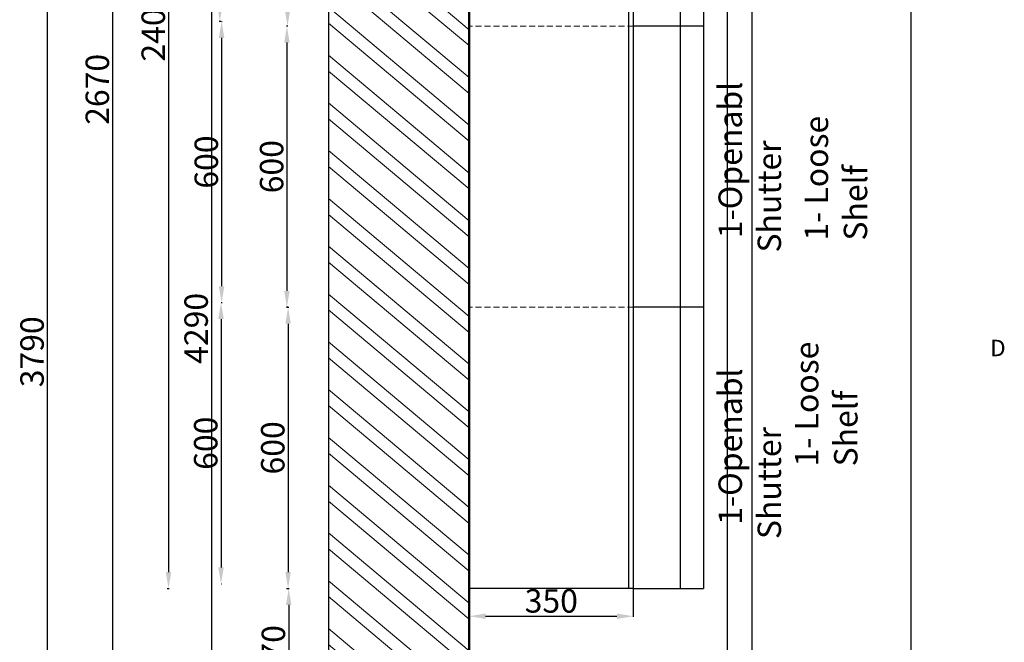
# Model space of a CAD drawing. Units: millimetres. Extents: x 407065 to 421840, y 1168257 to 1177792.
# Tile 4 of 17: x 407065 to 409166, y 1174623 to 1175951. Entities that reach past the tile are written whole.
import ezdxf

# ---------------------------------------------------------------- set-up
doc = ezdxf.new("R2010")
doc.units = ezdxf.units.MM
doc.linetypes.add('DASHED', pattern=[19.05, 12.7, -6.35])
for name, color, linetype, lineweight in [('A-ANNO-DIMS', 6, 'Continuous', 18), ('A-ANNO-TEXT', 30, 'Continuous', 18), ('A-FURN', 3, 'Continuous', 25), ('A-FURN-HIDN', 7, 'DASHED', 18), ('A-WALL', 7, 'Continuous', 50), ('A-WALL-PATT', 8, 'Continuous', 13)]:
    doc.layers.add(name, color=color, linetype=linetype, lineweight=lineweight)
doc.styles.get("Standard").update_dxf_attribs({"font": 'arial.ttf'})
doc.dimstyles.new('ISO-25', dxfattribs={"dimtxt": 50, "dimasz": 35, "dimexe": 1.25, "dimexo": 0.625, "dimtad": 1, "dimdec": 1, "dimtxsty": 'Standard', "dimcen": 35, "dimadec": 0, "dimazin": 0, "dimtfac": 1, "dimtdec": 1, "dimtmove": 0, "dimatfit": 3, "dimfxl": 1, "dimarcsym": 0})

# ---------------------------------------------------------------- blocks, each defined once
blk = doc.blocks.new('*D40')
at = {"layer": 'A-ANNO-DIMS', "color": 0, "lineweight": -2, "transparency": 16777216}
for p, q in [((407637.3, 1176347.8), (407635.4, 1176347.8)), ((407636.7, 1176312.8), (407636.7, 1175972.8)), ((407637.3, 1175937.8), (407635.4, 1175937.8))]:
    blk.add_line(p, q, dxfattribs=at)
at = {"layer": 'A-ANNO-DIMS', "color": 0, "transparency": 16777216}
for points in [[(407630.8, 1176312.8), (407642.5, 1176312.8), (407636.7, 1176347.8)], [(407630.8, 1175972.8), (407642.5, 1175972.8), (407636.7, 1175937.8)]]:
    blk.add_solid(points, dxfattribs=at)
at = {"layer": 'Defpoints', "color": 0, "transparency": 16777216}
for p in [(407637.9, 1176347.8), (407636.7, 1175937.8), (407637.9, 1175937.8)]:
    blk.add_point(p, dxfattribs=at)
at = {"layer": 'A-ANNO-DIMS', "color": 0, "transparency": 16777216, "insert": (407610.5, 1176142.8), "char_height": 50, "attachment_point": 5, "rotation": 90}
blk.add_mtext('410', dxfattribs=at)
blk = doc.blocks.new('*D41')
at = {"layer": 'A-ANNO-DIMS', "color": 0, "lineweight": -2, "transparency": 16777216}
for p, q in [((407637.3, 1175937.8), (407634.2, 1175937.8)), ((407635.4, 1175902.8), (407635.4, 1175372.8)), ((407637.3, 1175337.8), (407634.2, 1175337.8))]:
    blk.add_line(p, q, dxfattribs=at)
at = {"layer": 'A-ANNO-DIMS', "color": 0, "transparency": 16777216}
for points in [[(407629.6, 1175902.8), (407641.2, 1175902.8), (407635.4, 1175937.8)], [(407629.6, 1175372.8), (407641.2, 1175372.8), (407635.4, 1175337.8)]]:
    blk.add_solid(points, dxfattribs=at)
at = {"layer": 'Defpoints', "color": 0, "transparency": 16777216}
for p in [(407637.9, 1175937.8), (407635.4, 1175337.8), (407637.9, 1175337.8)]:
    blk.add_point(p, dxfattribs=at)
at = {"layer": 'A-ANNO-DIMS', "color": 0, "transparency": 16777216, "insert": (407609.2, 1175637.8), "char_height": 50, "attachment_point": 5, "rotation": 90}
blk.add_mtext('600', dxfattribs=at)
blk = doc.blocks.new('*D42')
at = {"layer": 'A-ANNO-DIMS', "color": 0, "lineweight": -2, "transparency": 16777216}
for p, q in [((407634.8, 1175337.8), (407639.2, 1175337.8)), ((407637.9, 1175302.8), (407637.9, 1174772.8)), ((407634.8, 1174737.8), (407639.2, 1174737.8))]:
    blk.add_line(p, q, dxfattribs=at)
at = {"layer": 'A-ANNO-DIMS', "color": 0, "transparency": 16777216}
for points in [[(407632.1, 1175302.8), (407643.7, 1175302.8), (407637.9, 1175337.8)], [(407632.1, 1174772.8), (407643.7, 1174772.8), (407637.9, 1174737.8)]]:
    blk.add_solid(points, dxfattribs=at)
at = {"layer": 'Defpoints', "color": 0, "transparency": 16777216}
for p in [(407634.2, 1175337.8), (407634.2, 1174737.8), (407637.9, 1174737.8)]:
    blk.add_point(p, dxfattribs=at)
at = {"layer": 'A-ANNO-DIMS', "color": 0, "transparency": 16777216, "insert": (407611.7, 1175037.8), "char_height": 50, "attachment_point": 5, "rotation": 90}
blk.add_mtext('600', dxfattribs=at)
blk = doc.blocks.new('*D43')
at = {"layer": 'A-ANNO-DIMS', "color": 0, "lineweight": -2, "transparency": 16777216}
for p, q in [((407635.4, 1174737.8), (407640.4, 1174737.8)), ((407639.2, 1174702.8), (407639.2, 1174502.8)), ((407635.4, 1174467.8), (407640.4, 1174467.8))]:
    blk.add_line(p, q, dxfattribs=at)
at = {"layer": 'A-ANNO-DIMS', "color": 0, "transparency": 16777216}
for points in [[(407633.3, 1174702.8), (407645, 1174702.8), (407639.2, 1174737.8)], [(407633.3, 1174502.8), (407645, 1174502.8), (407639.2, 1174467.8)]]:
    blk.add_solid(points, dxfattribs=at)
at = {"layer": 'Defpoints', "color": 0, "transparency": 16777216}
for p in [(407634.8, 1174737.8), (407634.8, 1174467.8), (407639.2, 1174467.8)]:
    blk.add_point(p, dxfattribs=at)
at = {"layer": 'A-ANNO-DIMS', "color": 0, "transparency": 16777216, "insert": (407613, 1174602.8), "char_height": 50, "attachment_point": 5, "rotation": 90}
blk.add_mtext('270', dxfattribs=at)
blk = doc.blocks.new('*D46')
at = {"layer": 'A-ANNO-DIMS', "color": 0, "lineweight": -2, "transparency": 16777216}
for p, q in [((407495.4, 1176497.7), (407491.1, 1176497.7)), ((407492.3, 1176462.7), (407492.3, 1175982.7)), ((407495.4, 1175947.7), (407491.1, 1175947.7))]:
    blk.add_line(p, q, dxfattribs=at)
at = {"layer": 'A-ANNO-DIMS', "color": 0, "transparency": 16777216}
for points in [[(407486.5, 1176462.7), (407498.2, 1176462.7), (407492.3, 1176497.7)], [(407486.5, 1175982.7), (407498.2, 1175982.7), (407492.3, 1175947.7)]]:
    blk.add_solid(points, dxfattribs=at)
at = {"layer": 'Defpoints', "color": 0, "transparency": 16777216}
for p in [(407496.1, 1176497.7), (407492.3, 1175947.7), (407496.1, 1175947.7)]:
    blk.add_point(p, dxfattribs=at)
at = {"layer": 'A-ANNO-DIMS', "color": 0, "transparency": 16777216, "insert": (407466.2, 1176222.7), "char_height": 50, "attachment_point": 5, "rotation": 90}
blk.add_mtext('550', dxfattribs=at)
blk = doc.blocks.new('*D47')
at = {"layer": 'A-ANNO-DIMS', "color": 0, "lineweight": -2, "transparency": 16777216}
for p, q in [((407496.7, 1175947.7), (407497.3, 1175947.7)), ((407496.1, 1175912.7), (407496.1, 1175382.7)), ((407496.7, 1175347.7), (407497.3, 1175347.7))]:
    blk.add_line(p, q, dxfattribs=at)
at = {"layer": 'A-ANNO-DIMS', "color": 0, "transparency": 16777216}
for points in [[(407490.2, 1175912.7), (407501.9, 1175912.7), (407496.1, 1175947.7)], [(407490.2, 1175382.7), (407501.9, 1175382.7), (407496.1, 1175347.7)]]:
    blk.add_solid(points, dxfattribs=at)
at = {"layer": 'Defpoints', "color": 0, "transparency": 16777216}
for p in [(407496.1, 1175947.7), (407496.1, 1175347.7), (407496.1, 1175347.7)]:
    blk.add_point(p, dxfattribs=at)
at = {"layer": 'A-ANNO-DIMS', "color": 0, "transparency": 16777216, "insert": (407469.9, 1175647.7), "char_height": 50, "attachment_point": 5, "rotation": 90}
blk.add_mtext('600', dxfattribs=at)
blk = doc.blocks.new('*D48')
at = {"layer": 'A-ANNO-DIMS', "color": 0, "lineweight": -2, "transparency": 16777216}
for p, q in [((407495.4, 1175347.7), (407496.1, 1175347.7)), ((407494.8, 1175312.7), (407494.8, 1174782.7)), ((407495.4, 1174747.7), (407496.1, 1174747.7))]:
    blk.add_line(p, q, dxfattribs=at)
at = {"layer": 'A-ANNO-DIMS', "color": 0, "transparency": 16777216}
for points in [[(407489, 1175312.7), (407500.7, 1175312.7), (407494.8, 1175347.7)], [(407489, 1174782.7), (407500.7, 1174782.7), (407494.8, 1174747.7)]]:
    blk.add_solid(points, dxfattribs=at)
at = {"layer": 'Defpoints', "color": 0, "transparency": 16777216}
for p in [(407494.8, 1175347.7), (407494.8, 1174747.7), (407494.8, 1174747.7)]:
    blk.add_point(p, dxfattribs=at)
at = {"layer": 'A-ANNO-DIMS', "color": 0, "transparency": 16777216, "insert": (407468.7, 1175047.7), "char_height": 50, "attachment_point": 5, "rotation": 90}
blk.add_mtext('600', dxfattribs=at)
blk = doc.blocks.new('*D49')
at = {"layer": 'A-ANNO-DIMS', "color": 0, "lineweight": -2, "transparency": 16777216}
for p, q in [((407380.2, 1177137.8), (407384.1, 1177137.8)), ((407382.9, 1177102.8), (407382.9, 1174772.8)), ((407380.2, 1174737.8), (407384.1, 1174737.8))]:
    blk.add_line(p, q, dxfattribs=at)
at = {"layer": 'A-ANNO-DIMS', "color": 0, "transparency": 16777216}
for points in [[(407377, 1177102.8), (407388.7, 1177102.8), (407382.9, 1177137.8)], [(407377, 1174772.8), (407388.7, 1174772.8), (407382.9, 1174737.8)]]:
    blk.add_solid(points, dxfattribs=at)
at = {"layer": 'Defpoints', "color": 0, "transparency": 16777216}
for p in [(407379.6, 1177137.8), (407379.6, 1174737.8), (407382.9, 1174737.8)]:
    blk.add_point(p, dxfattribs=at)
at = {"layer": 'A-ANNO-DIMS', "color": 0, "transparency": 16777216, "insert": (407356.7, 1175937.8), "char_height": 50, "attachment_point": 5, "rotation": 90}
blk.add_mtext('2400', dxfattribs=at)
blk = doc.blocks.new('*D50')
at = {"layer": 'A-ANNO-DIMS', "color": 0, "lineweight": -2, "transparency": 16777216}
for p, q in [((407237.7, 1177137.8), (407264.8, 1177137.8)), ((407263.5, 1177102.8), (407263.5, 1174502.8)), ((407237.7, 1174467.8), (407264.8, 1174467.8))]:
    blk.add_line(p, q, dxfattribs=at)
at = {"layer": 'A-ANNO-DIMS', "color": 0, "transparency": 16777216}
for points in [[(407257.7, 1177102.8), (407269.4, 1177102.8), (407263.5, 1177137.8)], [(407257.7, 1174502.8), (407269.4, 1174502.8), (407263.5, 1174467.8)]]:
    blk.add_solid(points, dxfattribs=at)
at = {"layer": 'Defpoints', "color": 0, "transparency": 16777216}
for p in [(407237, 1177137.8), (407237, 1174467.8), (407263.5, 1174467.8)]:
    blk.add_point(p, dxfattribs=at)
at = {"layer": 'A-ANNO-DIMS', "color": 0, "transparency": 16777216, "insert": (407237.4, 1175802.8), "char_height": 50, "attachment_point": 5, "rotation": 90}
blk.add_mtext('2670', dxfattribs=at)
blk = doc.blocks.new('*D51')
at = {"layer": 'A-ANNO-DIMS', "color": 0, "lineweight": -2, "transparency": 16777216}
for p, q in [((407115, 1177137.8), (407125.6, 1177137.8)), ((407124.3, 1177102.8), (407124.3, 1173382.8)), ((407115, 1173347.8), (407125.6, 1173347.8))]:
    blk.add_line(p, q, dxfattribs=at)
at = {"layer": 'A-ANNO-DIMS', "color": 0, "transparency": 16777216}
for points in [[(407118.5, 1177102.8), (407130.2, 1177102.8), (407124.3, 1177137.8)], [(407118.5, 1173382.8), (407130.2, 1173382.8), (407124.3, 1173347.8)]]:
    blk.add_solid(points, dxfattribs=at)
at = {"layer": 'Defpoints', "color": 0, "transparency": 16777216}
for p in [(407114.4, 1177137.8), (407114.4, 1173347.8), (407124.3, 1173347.8)]:
    blk.add_point(p, dxfattribs=at)
at = {"layer": 'A-ANNO-DIMS', "color": 0, "transparency": 16777216, "insert": (407098.2, 1175242.8), "char_height": 50, "attachment_point": 5, "rotation": 90}
blk.add_mtext('3790', dxfattribs=at)
blk = doc.blocks.new('*D53')
at = {"layer": 'A-ANNO-DIMS', "color": 0, "lineweight": -2, "transparency": 16777216}
for p, q in [((408024.3, 1174737.2), (408024.3, 1174677.2)), ((408374.3, 1174737.2), (408374.3, 1174677.2)), ((408059.3, 1174678.5), (408339.3, 1174678.5))]:
    blk.add_line(p, q, dxfattribs=at)
at = {"layer": 'A-ANNO-DIMS', "color": 0, "transparency": 16777216}
for points in [[(408059.3, 1174684.3), (408059.3, 1174672.7), (408024.3, 1174678.5)], [(408339.3, 1174684.3), (408339.3, 1174672.7), (408374.3, 1174678.5)]]:
    blk.add_solid(points, dxfattribs=at)
at = {"layer": 'Defpoints', "color": 0, "transparency": 16777216}
for p in [(408024.3, 1174737.8), (408374.3, 1174737.8), (408374.3, 1174678.5)]:
    blk.add_point(p, dxfattribs=at)
at = {"layer": 'A-ANNO-DIMS', "color": 0, "transparency": 16777216, "insert": (408199.3, 1174704.7), "char_height": 50, "attachment_point": 5}
blk.add_mtext('350', dxfattribs=at)
blk = doc.blocks.new('*D166')
at = {"layer": 'A-ANNO-DIMS', "color": 0, "lineweight": -2, "transparency": 16777216}
for p, q in [((407723.7, 1177437.8), (407473.1, 1177437.8)), ((407474.3, 1177402.8), (407474.3, 1173182.8)), ((407723.7, 1173147.8), (407473.1, 1173147.8))]:
    blk.add_line(p, q, dxfattribs=at)
at = {"layer": 'A-ANNO-DIMS', "color": 0, "transparency": 16777216}
for points in [[(407468.5, 1177402.8), (407480.1, 1177402.8), (407474.3, 1177437.8)], [(407468.5, 1173182.8), (407480.1, 1173182.8), (407474.3, 1173147.8)]]:
    blk.add_solid(points, dxfattribs=at)
at = {"layer": 'Defpoints', "color": 0, "transparency": 16777216}
for p in [(407724.3, 1177437.8), (407474.3, 1173147.8), (407724.3, 1173147.8)]:
    blk.add_point(p, dxfattribs=at)
at = {"layer": 'A-ANNO-DIMS', "color": 0, "transparency": 16777216, "insert": (407448.2, 1175292.8), "char_height": 50, "attachment_point": 5, "rotation": 90}
blk.add_mtext('4290', dxfattribs=at)
blk = doc.blocks.new('*D174')
at = {"layer": 'A-ANNO-DIMS', "color": 0, "lineweight": -2, "transparency": 16777216}
for p, q in [((408627.4, 1176861), (408627.4, 1172896.5)), ((408966, 1176861), (408966, 1172896.5)), ((408662.4, 1172897.8), (408931, 1172897.8))]:
    blk.add_line(p, q, dxfattribs=at)
at = {"layer": 'A-ANNO-DIMS', "color": 0, "transparency": 16777216}
for points in [[(408662.4, 1172903.6), (408662.4, 1172892), (408627.4, 1172897.8)], [(408931, 1172903.6), (408931, 1172892), (408966, 1172897.8)]]:
    blk.add_solid(points, dxfattribs=at)
at = {"layer": 'Defpoints', "color": 0, "transparency": 16777216}
for p in [(408627.4, 1176861.7), (408966, 1176861.7), (408966, 1172897.8)]:
    blk.add_point(p, dxfattribs=at)
at = {"layer": 'A-ANNO-DIMS', "color": 0, "transparency": 16777216, "insert": (408796.7, 1172924), "char_height": 50, "attachment_point": 5}
blk.add_mtext('338.63', dxfattribs=at)
blk = doc.blocks.new('*D176')
at = {"layer": 'A-ANNO-DIMS', "color": 0, "lineweight": -2, "transparency": 16777216}
for p, q in [((408574.3, 1176984.8), (408574.3, 1172896.5)), ((408627.4, 1176861), (408627.4, 1172896.5)), ((408539.3, 1172897.8), (408504.3, 1172897.8)), ((408574.3, 1172897.8), (408627.4, 1172897.8)), ((408662.4, 1172897.8), (408867.1, 1172897.8))]:
    blk.add_line(p, q, dxfattribs=at)
at = {"layer": 'A-ANNO-DIMS', "color": 0, "transparency": 16777216}
for points in [[(408539.3, 1172903.6), (408539.3, 1172892), (408574.3, 1172897.8)], [(408662.4, 1172903.6), (408662.4, 1172892), (408627.4, 1172897.8)]]:
    blk.add_solid(points, dxfattribs=at)
at = {"layer": 'Defpoints', "color": 0, "transparency": 16777216}
for p in [(408574.3, 1176985.5), (408627.4, 1176861.7), (408627.4, 1172897.8)]:
    blk.add_point(p, dxfattribs=at)
at = {"layer": 'A-ANNO-DIMS', "color": 0, "transparency": 16777216, "insert": (408782.2, 1172924), "char_height": 50, "attachment_point": 5}
blk.add_mtext('53.04', dxfattribs=at)

msp = doc.modelspace()

# ---------------------------------------------------------------- hatches: boundary and pattern name
at = {"layer": 'A-WALL-PATT'}
h = msp.add_hatch(dxfattribs=at)
h.set_pattern_fill('ANSI32', color=256, scale=8.2, angle=95)
h.paths.add_polyline_path([(408024.3133, 1177137.7952), (407724.3133, 1177137.7952), (407724.3133, 1174467.7952), (408024.3133, 1174467.7952)])

# ---------------------------------------------------------------- linework, layer by layer
at = {"layer": 'A-FURN'}
for p, q in [((407724.3133, 1177437.7952), (407724.3133, 1174467.7952)), ((408364.3133, 1177137.7952), (408364.3133, 1174737.7952)), ((408374.3133, 1177137.7952), (408374.3133, 1174737.7952)), ((408474.3133, 1177137.7952), (408474.3133, 1174737.7952)), ((408524.3133, 1177137.7952), (408524.3133, 1174737.7952)), ((408524.3133, 1175937.7952), (408374.3133, 1175937.7952)), ((408524.3133, 1175337.7952), (408374.3133, 1175337.7952)), ((408374.3133, 1174737.7952), (408024.3133, 1174737.7952)), ((408374.3133, 1174737.7952), (408524.3133, 1174737.7952))]:
    msp.add_line(p, q, dxfattribs=at)
at = {"layer": 'A-FURN-HIDN'}
for p, q in [((408374.3133, 1175937.7952), (408024.3133, 1175937.7952)), ((408374.3133, 1175337.7952), (408024.3133, 1175337.7952))]:
    msp.add_line(p, q, dxfattribs=at)
at = {"layer": 'A-WALL'}
msp.add_line((408024.3133, 1177137.7952), (408024.3133, 1174467.7952), dxfattribs=at)

# ---------------------------------------------------------------- texts
at = {"layer": 'A-ANNO-TEXT', "char_height": 50, "attachment_point": 1, "rotation": 90}
for s, width, insert in [('  1-Openabl Shutter', 455.344125, (408556.0224, 1175454.691)), ('1- Loose Shelf', 382.409863, (408739.8015, 1175480.1308)), ('1- Loose Shelf', 382.409863, (408719.1388, 1174998.2143)), ('  1-Openabl Shutter', 527.083716, (408556.0224, 1174843.1115))]:
    msp.add_mtext_dynamic_manual_height_columns(s, width=width, gutter_width=12.5, heights=[0], dxfattribs=dict(at, insert=insert))
at = {"layer": 'A-ANNO-TEXT', "insert": (409135.6345, 1175268.3838), "char_height": 35, "attachment_point": 1}
msp.add_mtext_dynamic_manual_height_columns('D', width=382.409863, gutter_width=12.5, heights=[0], dxfattribs=at)

# ---------------------------------------------------------------- dimensions: what is measured, and where the dimension line sits
at = {"layer": 'A-ANNO-DIMS'}
for base, p1, p2, override, picture, middle in [((407474.3133, 1173147.7952), (407724.3133, 1177437.7952), (407724.3133, 1173147.7952), {"dimdec": 0, "dimlfac": 1, "dimrnd": 0, "dimzin": 0, "dimdsep": 46, "dimlunit": 2}, '*D166', (407448.1597, 1175292.7952)), ((407124.3456, 1173347.7952), (407114.4021, 1177137.7952), (407114.4021, 1173347.7952), {"dimclrd": 0, "dimclre": 0, "dimclrt": 0}, '*D51', (407098.1749, 1175242.7952)), ((407263.5498, 1174467.7952), (407237.0345, 1177137.7952), (407237.0345, 1174467.7952), {"dimclrd": 0, "dimclre": 0, "dimclrt": 0}, '*D50', (407237.3961, 1175802.7952)), ((407382.8674, 1174737.7952), (407379.577, 1177137.7952), (407379.577, 1174737.7952), {"dimclrd": 0, "dimclre": 0, "dimclrt": 0}, '*D49', (407356.7137, 1175937.7952)), ((407492.3211, 1175947.6795), (407496.0711, 1176497.6795), (407496.0711, 1175947.6795), {"dimclrd": 0, "dimclre": 0, "dimclrt": 0}, '*D46', (407466.1675, 1176222.6795)), ((407636.652, 1175937.7952), (407637.902, 1176347.7952), (407637.902, 1175937.7952), {"dimclrd": 0, "dimclre": 0, "dimclrt": 0}, '*D40', (407610.4983, 1176142.7952)), ((407496.0711, 1175347.6795), (407496.0711, 1175947.6795), (407496.0711, 1175347.6795), {"dimclrd": 0, "dimclre": 0, "dimclrt": 0}, '*D47', (407469.9175, 1175647.6795)), ((407635.402, 1175337.7952), (407637.902, 1175937.7952), (407637.902, 1175337.7952), {"dimclrd": 0, "dimclre": 0, "dimclrt": 0}, '*D41', (407609.2483, 1175637.7952)), ((407494.8211, 1174747.6795), (407494.8211, 1175347.6795), (407494.8211, 1174747.6795), {"dimclrd": 0, "dimclre": 0, "dimclrt": 0}, '*D48', (407468.6675, 1175047.6795)), ((407637.902, 1174737.7952), (407634.152, 1175337.7952), (407634.152, 1174737.7952), {"dimclrd": 0, "dimclre": 0, "dimclrt": 0}, '*D42', (407611.7483, 1175037.7952)), ((407639.152, 1174467.7952), (407634.777, 1174737.7952), (407634.777, 1174467.7952), {"dimclrd": 0, "dimclre": 0, "dimclrt": 0}, '*D43', (407612.9983, 1174602.7952))]:
    dim = msp.add_linear_dim(base=base, p1=p1, p2=p2, angle=90, dimstyle='ISO-25', override=override, dxfattribs=at)
    dim.commit()
    dim.dimension.update_dxf_attribs({"geometry": picture, "text_midpoint": middle})
for base, p1, p2, override, picture, middle in [((408627.3554, 1172897.7952), (408574.3133, 1176985.4747), (408627.3554, 1176861.6588), {"dimdec": 2, "dimlfac": 1, "dimrnd": 0, "dimzin": 0, "dimdsep": 46, "dimlunit": 2}, '*D176', (408782.2403, 1172923.9659)), ((408965.99043, 1172897.79525), (408627.35545, 1176861.65877), (408965.99043, 1176861.65877), {"dimdec": 2, "dimlfac": 1, "dimrnd": 0, "dimzin": 0, "dimdsep": 46, "dimlunit": 2}, '*D174', (408796.67294, 1172923.96595)), ((408374.3133, 1174678.4967), (408024.3133, 1174737.7952), (408374.3133, 1174737.7952), {"dimclrd": 0, "dimclre": 0, "dimclrt": 0}, '*D53', (408199.3133, 1174704.6674))]:
    dim = msp.add_linear_dim(base=base, p1=p1, p2=p2, dimstyle='ISO-25', override=override, dxfattribs=at)
    dim.commit()
    dim.dimension.update_dxf_attribs({"geometry": picture, "text_midpoint": middle})

doc.saveas('drawing.dxf')
